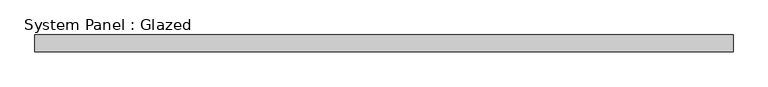
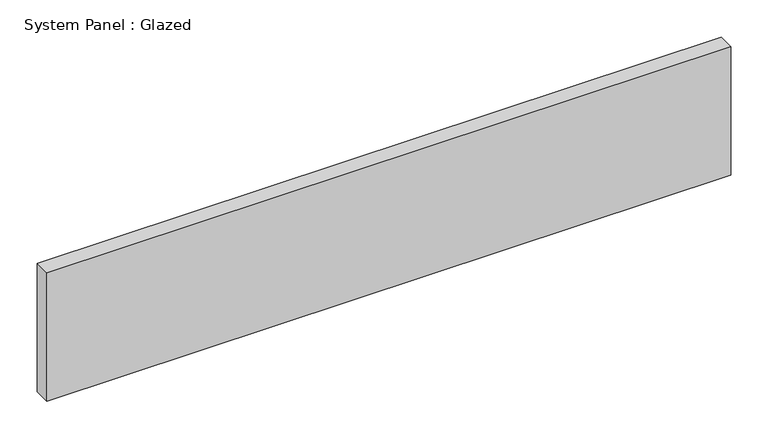
"""IFC4 building model written with IfcOpenShell, lengths in millimetres: plate geometry, System Panel : Glazed."""

from ifc_helpers import new_model, si_unit, origin, origin_with_axes, place, context, project, spatial, polyline, outline, extrude, source, transform, mapped, element, save


def system_panel_glazed_b341651b(model_context):
    return source(origin(), model_context, "Body", "SweptSolid", [
        extrude(outline(polyline([(527.05, 19.05), (-527.05, 19.05), (-527.05, 44.45), (527.05, 44.45), (527.05, 19.05)])), origin_with_axes(), (0.0, 0.0, 1.0), 209.55),
    ])


if __name__ == "__main__":
    model = new_model("IFC4")
    model_context = context("Model", 3, world=origin())
    ifc_project = project(units=[si_unit("LENGTHUNIT", "METRE", prefix="MILLI")], contexts=[model_context])
    site = spatial("IfcSite", under=ifc_project)
    building = spatial("IfcBuilding", under=site)
    placement = place(None, origin())
    system_panel_glazed_shape = system_panel_glazed_b341651b(model_context)
    element("IfcPlate", 1, ObjectType="System Panel : Glazed", at=placement, inside=building, context=model_context, shape_type="MappedRepresentation", body=[
        mapped(system_panel_glazed_shape, transform((0.0, 0.0, 0.0), x_axis=(1.0, 0.0, 0.0), y_axis=(0.0, 1.0, 0.0), z_axis=(0.0, 0.0, 1.0))),
    ])
    save(model, "model.ifc")

# Revit data of these elements
# Type "System Panel : Glazed"
#   Construction Type Id = "GSP4R"
#   Analytic Construction = "1/8 in Pilkington single glazing"
#   Visual Light Transmittance = 0.9
#   Solar Heat Gain Coefficient = 0.86
#   Heat Transfer Coefficient (U) = 1.18115 BTU/(h·ft²·°F)
#   Define Thermal Properties by = 1
# Element 1 (IfcPlate, "System Panel : Glazed")
#   Materials on its faces: "Glass"
# Materials
#   "Glass": class "Glass", colour RGB 0 128 192, transparency 0.75, Description = "Soda Lime Glass", Cost = 0
